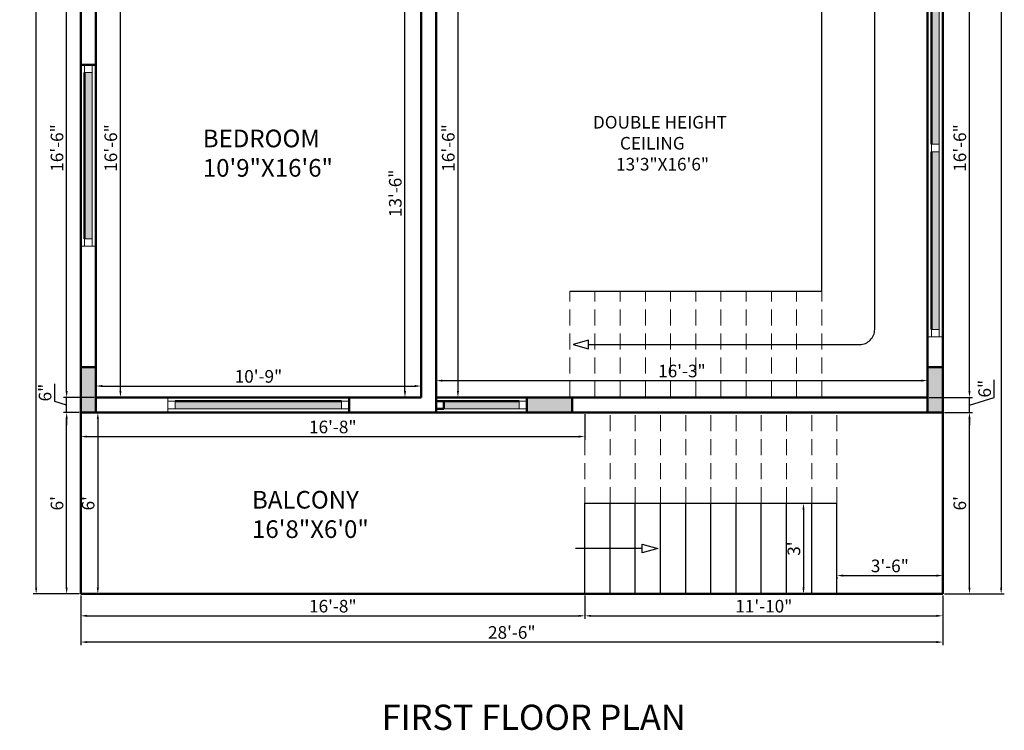
# Model space of a CAD drawing. Units: inches. Extents: x 3064 to 19385, y 846 to 15425.
# Tile 53 of 108: x 6445 to 6835, y 850 to 1132. Entities that reach past the tile are written whole.
import ezdxf

# ---------------------------------------------------------------- set-up
doc = ezdxf.new("R2010")
doc.units = ezdxf.units.IN
doc.linetypes.add('DASHED', pattern=[19.05, 12.7, -6.35])
for name, color, linetype, lineweight in [('A-ANNO-DIMS', 2, 'Continuous', 18), ('A-ANNO-TEXT', 7, 'Continuous', 25), ('A-AREA-IDEN', 3, 'Continuous', 18), ('A-COLS', 1, 'Continuous', 35), ('A-FLOR-STRS', 2, 'Continuous', 25), ('A-FLOR-STRS-OVHD', 2, 'DASHED', 18), ('A-GLAZ', 4, 'Continuous', 18), ('A-WALL', 7, 'Continuous', 50)]:
    doc.layers.add(name, color=color, linetype=linetype, lineweight=lineweight)
doc.styles.get("Standard").update_dxf_attribs({"font": 'arial.ttf'})
doc.dimstyles.new('ISO-25', dxfattribs={"dimtxt": 9, "dimasz": 2.5, "dimexe": 1.25, "dimexo": 0.625, "dimtad": 1, "dimdec": 1, "dimlunit": 3, "dimtxsty": 'Standard', "dimcen": 2.5, "dimadec": 0, "dimazin": 0, "dimtfac": 1, "dimtdec": 1, "dimtmove": 0, "dimatfit": 3, "dimfxl": 1, "dimarcsym": 0})

# ---------------------------------------------------------------- blocks, each defined once
blk = doc.blocks.new('*D135')
at = {"layer": 'A-ANNO-DIMS', "color": 0, "lineweight": -2, "transparency": 16777216}
for p, q in [((6468.41, 976.34), (6462.18, 976.34)), ((6463.43, 906.84), (6463.43, 973.84)), ((6468.41, 904.34), (6462.18, 904.34))]:
    blk.add_line(p, q, dxfattribs=at)
at = {"layer": 'A-ANNO-DIMS', "color": 0, "transparency": 16777216}
for points in [[(6463.02, 973.84), (6463.85, 973.84), (6463.43, 976.34)], [(6463.02, 906.84), (6463.85, 906.84), (6463.43, 904.34)]]:
    blk.add_solid(points, dxfattribs=at)
at = {"layer": 'Defpoints', "color": 0, "transparency": 16777216}
for p in [(6463.43, 976.34), (6469.03, 976.34), (6469.03, 904.34)]:
    blk.add_point(p, dxfattribs=at)
at = {"layer": 'A-ANNO-DIMS', "color": 0, "transparency": 16777216, "insert": (6460.26, 940.34), "char_height": 5, "attachment_point": 5, "rotation": 90}
blk.add_mtext("6'", dxfattribs=at)
blk = doc.blocks.new('*D127')
at = {"layer": 'A-ANNO-DIMS', "color": 0, "lineweight": -2, "transparency": 16777216}
for p, q in [((6458.69, 980.76), (6458.69, 987.79)), ((6463.43, 984.84), (6463.43, 987.34)), ((6463.43, 979.34), (6458.69, 980.76)), ((6474.41, 982.34), (6462.18, 982.34)), ((6463.43, 976.34), (6463.43, 982.34)), ((6463.43, 976.34), (6463.43, 982.34)), ((6468.41, 976.34), (6462.18, 976.34)), ((6463.43, 973.84), (6463.43, 971.34))]:
    blk.add_line(p, q, dxfattribs=at)
at = {"layer": 'A-ANNO-DIMS', "color": 0, "transparency": 16777216}
for points in [[(6463.02, 984.84), (6463.85, 984.84), (6463.43, 982.34)], [(6463.02, 973.84), (6463.85, 973.84), (6463.43, 976.34)]]:
    blk.add_solid(points, dxfattribs=at)
at = {"layer": 'Defpoints', "color": 0, "transparency": 16777216}
for p in [(6463.43, 982.34), (6475.03, 982.34), (6469.03, 976.34)]:
    blk.add_point(p, dxfattribs=at)
at = {"layer": 'A-ANNO-DIMS', "color": 0, "transparency": 16777216, "insert": (6455.52, 984.27), "char_height": 5, "attachment_point": 5, "rotation": 90}
blk.add_mtext('6"', dxfattribs=at)
blk = doc.blocks.new('*D128')
at = {"layer": 'A-ANNO-DIMS', "color": 0, "lineweight": -2, "transparency": 16777216}
for p, q in [((6474.41, 1180.34), (6462.18, 1180.34)), ((6463.43, 984.84), (6463.43, 1177.84)), ((6474.41, 982.34), (6462.18, 982.34))]:
    blk.add_line(p, q, dxfattribs=at)
at = {"layer": 'A-ANNO-DIMS', "color": 0, "transparency": 16777216}
for points in [[(6463.02, 1177.84), (6463.85, 1177.84), (6463.43, 1180.34)], [(6463.02, 984.84), (6463.85, 984.84), (6463.43, 982.34)]]:
    blk.add_solid(points, dxfattribs=at)
at = {"layer": 'Defpoints', "color": 0, "transparency": 16777216}
for p in [(6463.43, 1180.34), (6475.03, 1180.34), (6475.03, 982.34)]:
    blk.add_point(p, dxfattribs=at)
at = {"layer": 'A-ANNO-DIMS', "color": 0, "transparency": 16777216, "insert": (6460.26, 1081.34), "char_height": 5, "attachment_point": 5, "rotation": 90}
blk.add_mtext('16\'-6"', dxfattribs=at)
blk = doc.blocks.new('*D126')
at = {"layer": 'A-ANNO-DIMS', "color": 0, "lineweight": -2, "transparency": 16777216}
for p, q in [((6468.41, 1396.34), (6450.1, 1396.34)), ((6451.35, 906.84), (6451.35, 1393.84)), ((6468.41, 904.34), (6450.1, 904.34))]:
    blk.add_line(p, q, dxfattribs=at)
at = {"layer": 'A-ANNO-DIMS', "color": 0, "transparency": 16777216}
for points in [[(6450.94, 1393.84), (6451.77, 1393.84), (6451.35, 1396.34)], [(6450.94, 906.84), (6451.77, 906.84), (6451.35, 904.34)]]:
    blk.add_solid(points, dxfattribs=at)
at = {"layer": 'Defpoints', "color": 0, "transparency": 16777216}
for p in [(6451.35, 1396.34), (6469.03, 1396.34), (6469.03, 904.34)]:
    blk.add_point(p, dxfattribs=at)
at = {"layer": 'A-ANNO-DIMS', "color": 0, "transparency": 16777216, "insert": (6448.22, 1150.34), "char_height": 5, "attachment_point": 5, "rotation": 90}
blk.add_mtext("41'", dxfattribs=at)
blk = doc.blocks.new('*D115')
at = {"layer": 'A-ANNO-DIMS', "color": 0, "lineweight": -2, "transparency": 16777216}
for p, q in [((6469.03, 903.71), (6469.03, 894.42)), ((6669.03, 903.71), (6669.03, 894.42)), ((6471.53, 895.67), (6666.53, 895.67))]:
    blk.add_line(p, q, dxfattribs=at)
at = {"layer": 'A-ANNO-DIMS', "color": 0, "transparency": 16777216}
for points in [[(6471.53, 896.08), (6471.53, 895.25), (6469.03, 895.67)], [(6666.53, 896.08), (6666.53, 895.25), (6669.03, 895.67)]]:
    blk.add_solid(points, dxfattribs=at)
at = {"layer": 'Defpoints', "color": 0, "transparency": 16777216}
for p in [(6469.03, 904.34), (6669.03, 904.34), (6669.03, 895.67)]:
    blk.add_point(p, dxfattribs=at)
at = {"layer": 'A-ANNO-DIMS', "color": 0, "transparency": 16777216, "insert": (6569.03, 898.85), "char_height": 5, "attachment_point": 5}
blk.add_mtext('16\'-8"', dxfattribs=at)
blk = doc.blocks.new('*D116')
at = {"layer": 'A-ANNO-DIMS', "color": 0, "lineweight": -2, "transparency": 16777216}
for p, q in [((6669.03, 903.71), (6669.03, 894.42)), ((6811.03, 903.71), (6811.03, 894.42)), ((6671.53, 895.67), (6808.53, 895.67))]:
    blk.add_line(p, q, dxfattribs=at)
at = {"layer": 'A-ANNO-DIMS', "color": 0, "transparency": 16777216}
for points in [[(6671.53, 896.08), (6671.53, 895.25), (6669.03, 895.67)], [(6808.53, 896.08), (6808.53, 895.25), (6811.03, 895.67)]]:
    blk.add_solid(points, dxfattribs=at)
at = {"layer": 'Defpoints', "color": 0, "transparency": 16777216}
for p in [(6669.03, 904.34), (6811.03, 904.34), (6811.03, 895.67)]:
    blk.add_point(p, dxfattribs=at)
at = {"layer": 'A-ANNO-DIMS', "color": 0, "transparency": 16777216, "insert": (6740.03, 898.85), "char_height": 5, "attachment_point": 5}
blk.add_mtext('11\'-10"', dxfattribs=at)
blk = doc.blocks.new('*D98')
at = {"layer": 'A-ANNO-DIMS', "color": 0, "lineweight": -2, "transparency": 16777216}
for p, q in [((6469.03, 903.71), (6469.03, 884.01)), ((6811.03, 903.71), (6811.03, 884.01)), ((6808.53, 885.26), (6471.53, 885.26))]:
    blk.add_line(p, q, dxfattribs=at)
at = {"layer": 'A-ANNO-DIMS', "color": 0, "transparency": 16777216}
for points in [[(6471.53, 885.67), (6471.53, 884.84), (6469.03, 885.26)], [(6808.53, 885.67), (6808.53, 884.84), (6811.03, 885.26)]]:
    blk.add_solid(points, dxfattribs=at)
at = {"layer": 'Defpoints', "color": 0, "transparency": 16777216}
for p in [(6469.03, 904.34), (6811.03, 904.34), (6469.03, 885.26)]:
    blk.add_point(p, dxfattribs=at)
at = {"layer": 'A-ANNO-DIMS', "color": 0, "transparency": 16777216, "insert": (6640.03, 888.43), "char_height": 5, "attachment_point": 5}
blk.add_mtext('28\'-6"', dxfattribs=at)
blk = doc.blocks.new('*D117')
at = {"layer": 'A-ANNO-DIMS', "color": 0, "lineweight": -2, "transparency": 16777216}
for p, q in [((6811.66, 976.34), (6822.87, 976.34)), ((6821.62, 906.84), (6821.62, 973.84)), ((6811.66, 904.34), (6822.87, 904.34))]:
    blk.add_line(p, q, dxfattribs=at)
at = {"layer": 'A-ANNO-DIMS', "color": 0, "transparency": 16777216}
for points in [[(6821.2, 973.84), (6822.03, 973.84), (6821.62, 976.34)], [(6821.2, 906.84), (6822.03, 906.84), (6821.62, 904.34)]]:
    blk.add_solid(points, dxfattribs=at)
at = {"layer": 'Defpoints', "color": 0, "transparency": 16777216}
for p in [(6811.03, 976.34), (6821.62, 976.34), (6811.03, 904.34)]:
    blk.add_point(p, dxfattribs=at)
at = {"layer": 'A-ANNO-DIMS', "color": 0, "transparency": 16777216, "insert": (6818.44, 940.34), "char_height": 5, "attachment_point": 5, "rotation": 90}
blk.add_mtext("6'", dxfattribs=at)
blk = doc.blocks.new('*D118')
at = {"layer": 'A-ANNO-DIMS', "color": 0, "lineweight": -2, "transparency": 16777216}
for p, q in [((6831.46, 982.29), (6831.46, 989.32)), ((6821.62, 984.84), (6821.62, 987.34)), ((6805.66, 982.34), (6822.87, 982.34)), ((6821.62, 976.34), (6821.62, 982.34)), ((6821.62, 976.34), (6821.62, 982.34)), ((6821.62, 979.34), (6831.46, 982.29)), ((6811.66, 976.34), (6822.87, 976.34)), ((6821.62, 973.84), (6821.62, 971.34))]:
    blk.add_line(p, q, dxfattribs=at)
at = {"layer": 'A-ANNO-DIMS', "color": 0, "transparency": 16777216}
for points in [[(6821.2, 984.84), (6822.03, 984.84), (6821.62, 982.34)], [(6821.2, 973.84), (6822.03, 973.84), (6821.62, 976.34)]]:
    blk.add_solid(points, dxfattribs=at)
at = {"layer": 'Defpoints', "color": 0, "transparency": 16777216}
for p in [(6805.03, 982.34), (6821.62, 982.34), (6811.03, 976.34)]:
    blk.add_point(p, dxfattribs=at)
at = {"layer": 'A-ANNO-DIMS', "color": 0, "transparency": 16777216, "insert": (6828.28, 985.81), "char_height": 5, "attachment_point": 5, "rotation": 90}
blk.add_mtext('6"', dxfattribs=at)
blk = doc.blocks.new('*D119')
at = {"layer": 'A-ANNO-DIMS', "color": 0, "lineweight": -2, "transparency": 16777216}
for p, q in [((6811.66, 1180.34), (6822.87, 1180.34)), ((6821.62, 984.84), (6821.62, 1177.84)), ((6805.66, 982.34), (6822.87, 982.34))]:
    blk.add_line(p, q, dxfattribs=at)
at = {"layer": 'A-ANNO-DIMS', "color": 0, "transparency": 16777216}
for points in [[(6821.2, 1177.84), (6822.03, 1177.84), (6821.62, 1180.34)], [(6821.2, 984.84), (6822.03, 984.84), (6821.62, 982.34)]]:
    blk.add_solid(points, dxfattribs=at)
at = {"layer": 'Defpoints', "color": 0, "transparency": 16777216}
for p in [(6811.03, 1180.34), (6821.62, 1180.34), (6805.03, 982.34)]:
    blk.add_point(p, dxfattribs=at)
at = {"layer": 'A-ANNO-DIMS', "color": 0, "transparency": 16777216, "insert": (6818.44, 1081.34), "char_height": 5, "attachment_point": 5, "rotation": 90}
blk.add_mtext('16\'-6"', dxfattribs=at)
blk = doc.blocks.new('*D104')
at = {"layer": 'A-ANNO-DIMS', "color": 0, "lineweight": -2, "transparency": 16777216}
for p, q in [((6811.66, 1396.34), (6835.44, 1396.34)), ((6834.19, 1393.84), (6834.19, 906.84)), ((6811.66, 904.34), (6835.44, 904.34))]:
    blk.add_line(p, q, dxfattribs=at)
at = {"layer": 'A-ANNO-DIMS', "color": 0, "transparency": 16777216}
for points in [[(6833.77, 1393.84), (6834.6, 1393.84), (6834.19, 1396.34)], [(6833.77, 906.84), (6834.6, 906.84), (6834.19, 904.34)]]:
    blk.add_solid(points, dxfattribs=at)
at = {"layer": 'Defpoints', "color": 0, "transparency": 16777216}
for p in [(6811.03, 1396.34), (6811.03, 904.34), (6834.19, 904.34)]:
    blk.add_point(p, dxfattribs=at)
at = {"layer": 'A-ANNO-DIMS', "color": 0, "transparency": 16777216, "insert": (6831.05, 1150.34), "char_height": 5, "attachment_point": 5, "rotation": 90}
blk.add_mtext("41'", dxfattribs=at)
blk = doc.blocks.new('*D181')
at = {"layer": 'A-ANNO-DIMS', "color": 0, "lineweight": -2, "transparency": 16777216}
for p, q in [((6469.03, 975.71), (6469.03, 965.55)), ((6669.03, 975.71), (6669.03, 965.55)), ((6471.53, 966.8), (6666.53, 966.8))]:
    blk.add_line(p, q, dxfattribs=at)
at = {"layer": 'A-ANNO-DIMS', "color": 0, "transparency": 16777216}
for points in [[(6471.53, 967.22), (6471.53, 966.39), (6469.03, 966.8)], [(6666.53, 967.22), (6666.53, 966.39), (6669.03, 966.8)]]:
    blk.add_solid(points, dxfattribs=at)
at = {"layer": 'Defpoints', "color": 0, "transparency": 16777216}
for p in [(6469.03, 976.34), (6669.03, 976.34), (6669.03, 966.8)]:
    blk.add_point(p, dxfattribs=at)
at = {"layer": 'A-ANNO-DIMS', "color": 0, "transparency": 16777216, "insert": (6569.03, 969.98), "char_height": 5, "attachment_point": 5}
blk.add_mtext('16\'-8"', dxfattribs=at)
blk = doc.blocks.new('*D182')
at = {"layer": 'A-ANNO-DIMS', "color": 0, "lineweight": -2, "transparency": 16777216}
for p, q in [((6469.66, 976.34), (6477.06, 976.34)), ((6475.81, 973.84), (6475.81, 906.84)), ((6469.66, 904.34), (6477.06, 904.34))]:
    blk.add_line(p, q, dxfattribs=at)
at = {"layer": 'A-ANNO-DIMS', "color": 0, "transparency": 16777216}
for points in [[(6475.39, 973.84), (6476.23, 973.84), (6475.81, 976.34)], [(6475.39, 906.84), (6476.23, 906.84), (6475.81, 904.34)]]:
    blk.add_solid(points, dxfattribs=at)
at = {"layer": 'Defpoints', "color": 0, "transparency": 16777216}
for p in [(6469.03, 976.34), (6469.03, 904.34), (6475.81, 904.34)]:
    blk.add_point(p, dxfattribs=at)
at = {"layer": 'A-ANNO-DIMS', "color": 0, "transparency": 16777216, "insert": (6472.63, 940.34), "char_height": 5, "attachment_point": 5, "rotation": 90}
blk.add_mtext("6'", dxfattribs=at)
blk = doc.blocks.new('*D183')
at = {"layer": 'A-ANNO-DIMS', "color": 0, "lineweight": -2, "transparency": 16777216}
for p, q in [((6769.03, 911.03), (6769.03, 910.4)), ((6771.53, 911.65), (6808.53, 911.65)), ((6811.03, 912.28), (6811.03, 912.9))]:
    blk.add_line(p, q, dxfattribs=at)
at = {"layer": 'A-ANNO-DIMS', "color": 0, "transparency": 16777216}
for points in [[(6771.53, 912.07), (6771.53, 911.23), (6769.03, 911.65)], [(6808.53, 912.07), (6808.53, 911.23), (6811.03, 911.65)]]:
    blk.add_solid(points, dxfattribs=at)
at = {"layer": 'Defpoints', "color": 0, "transparency": 16777216}
for p in [(6769.03, 911.65), (6811.03, 911.65), (6811.03, 911.65)]:
    blk.add_point(p, dxfattribs=at)
at = {"layer": 'A-ANNO-DIMS', "color": 0, "transparency": 16777216, "insert": (6790.03, 914.83), "char_height": 5, "attachment_point": 5}
blk.add_mtext('3\'-6"', dxfattribs=at)
blk = doc.blocks.new('*D184')
at = {"layer": 'A-ANNO-DIMS', "color": 0, "lineweight": -2, "transparency": 16777216}
for p, q in [((6754.21, 940.34), (6757.03, 940.34)), ((6755.78, 937.84), (6755.78, 906.84)), ((6754.21, 904.34), (6757.03, 904.34))]:
    blk.add_line(p, q, dxfattribs=at)
at = {"layer": 'A-ANNO-DIMS', "color": 0, "transparency": 16777216}
for points in [[(6755.36, 937.84), (6756.19, 937.84), (6755.78, 940.34)], [(6755.36, 906.84), (6756.19, 906.84), (6755.78, 904.34)]]:
    blk.add_solid(points, dxfattribs=at)
at = {"layer": 'Defpoints', "color": 0, "transparency": 16777216}
for p in [(6753.58, 940.34), (6753.58, 904.34), (6755.78, 904.34)]:
    blk.add_point(p, dxfattribs=at)
at = {"layer": 'A-ANNO-DIMS', "color": 0, "transparency": 16777216, "insert": (6752.6, 922.34), "char_height": 5, "attachment_point": 5, "rotation": 90}
blk.add_mtext("3'", dxfattribs=at)
blk = doc.blocks.new('*D187')
at = {"layer": 'A-ANNO-DIMS', "color": 0, "lineweight": -2, "transparency": 16777216}
for p, q in [((6475.03, 982.96), (6475.03, 988.12)), ((6477.53, 986.87), (6601.53, 986.87)), ((6604.03, 982.96), (6604.03, 988.12))]:
    blk.add_line(p, q, dxfattribs=at)
at = {"layer": 'A-ANNO-DIMS', "color": 0, "transparency": 16777216}
for points in [[(6477.53, 987.29), (6477.53, 986.45), (6475.03, 986.87)], [(6601.53, 987.29), (6601.53, 986.45), (6604.03, 986.87)]]:
    blk.add_solid(points, dxfattribs=at)
at = {"layer": 'Defpoints', "color": 0, "transparency": 16777216}
for p in [(6604.03, 986.87), (6475.03, 982.34), (6604.03, 982.34)]:
    blk.add_point(p, dxfattribs=at)
at = {"layer": 'A-ANNO-DIMS', "color": 0, "transparency": 16777216, "insert": (6539.53, 990.05), "char_height": 5, "attachment_point": 5}
blk.add_mtext('10\'-9"', dxfattribs=at)
blk = doc.blocks.new('*D188')
at = {"layer": 'A-ANNO-DIMS', "color": 0, "lineweight": -2, "transparency": 16777216}
for p, q in [((6475.66, 1180.34), (6486.03, 1180.34)), ((6484.78, 984.84), (6484.78, 1177.84)), ((6475.66, 982.34), (6486.03, 982.34))]:
    blk.add_line(p, q, dxfattribs=at)
at = {"layer": 'A-ANNO-DIMS', "color": 0, "transparency": 16777216}
for points in [[(6484.37, 1177.84), (6485.2, 1177.84), (6484.78, 1180.34)], [(6484.37, 984.84), (6485.2, 984.84), (6484.78, 982.34)]]:
    blk.add_solid(points, dxfattribs=at)
at = {"layer": 'Defpoints', "color": 0, "transparency": 16777216}
for p in [(6475.03, 1180.34), (6484.78, 1180.34), (6475.03, 982.34)]:
    blk.add_point(p, dxfattribs=at)
at = {"layer": 'A-ANNO-DIMS', "color": 0, "transparency": 16777216, "insert": (6481.6, 1081.34), "char_height": 5, "attachment_point": 5, "rotation": 90}
blk.add_mtext('16\'-6"', dxfattribs=at)
blk = doc.blocks.new('*D192')
at = {"layer": 'A-ANNO-DIMS', "color": 0, "lineweight": -2, "transparency": 16777216}
for p, q in [((6603.41, 1144.34), (6596.41, 1144.34)), ((6597.66, 984.84), (6597.66, 1141.84)), ((6603.41, 982.34), (6596.41, 982.34))]:
    blk.add_line(p, q, dxfattribs=at)
at = {"layer": 'A-ANNO-DIMS', "color": 0, "transparency": 16777216}
for points in [[(6597.25, 1141.84), (6598.08, 1141.84), (6597.66, 1144.34)], [(6597.25, 984.84), (6598.08, 984.84), (6597.66, 982.34)]]:
    blk.add_solid(points, dxfattribs=at)
at = {"layer": 'Defpoints', "color": 0, "transparency": 16777216}
for p in [(6597.66, 1144.34), (6604.03, 1144.34), (6604.03, 982.34)]:
    blk.add_point(p, dxfattribs=at)
at = {"layer": 'A-ANNO-DIMS', "color": 0, "transparency": 16777216, "insert": (6594.48, 1063.34), "char_height": 5, "attachment_point": 5, "rotation": 90}
blk.add_mtext('13\'-6"', dxfattribs=at)
blk = doc.blocks.new('*D216')
at = {"layer": 'A-ANNO-DIMS', "color": 0, "lineweight": -2, "transparency": 16777216}
for p, q in [((6610.66, 1180.34), (6619.92, 1180.34)), ((6618.67, 1177.84), (6618.67, 984.84)), ((6610.66, 982.34), (6619.92, 982.34))]:
    blk.add_line(p, q, dxfattribs=at)
at = {"layer": 'A-ANNO-DIMS', "color": 0, "transparency": 16777216}
for points in [[(6618.26, 1177.84), (6619.09, 1177.84), (6618.67, 1180.34)], [(6618.26, 984.84), (6619.09, 984.84), (6618.67, 982.34)]]:
    blk.add_solid(points, dxfattribs=at)
at = {"layer": 'Defpoints', "color": 0, "transparency": 16777216}
for p in [(6610.03, 1180.34), (6610.03, 982.34), (6618.67, 982.34)]:
    blk.add_point(p, dxfattribs=at)
at = {"layer": 'A-ANNO-DIMS', "color": 0, "transparency": 16777216, "insert": (6615.5, 1081.34), "char_height": 5, "attachment_point": 5, "rotation": 90}
blk.add_mtext('16\'-6"', dxfattribs=at)
blk = doc.blocks.new('*D217')
at = {"layer": 'A-ANNO-DIMS', "color": 0, "lineweight": -2, "transparency": 16777216}
for p, q in [((6610.03, 982.96), (6610.03, 990.26)), ((6612.53, 989.01), (6802.53, 989.01)), ((6805.03, 982.96), (6805.03, 990.26))]:
    blk.add_line(p, q, dxfattribs=at)
at = {"layer": 'A-ANNO-DIMS', "color": 0, "transparency": 16777216}
for points in [[(6612.53, 989.43), (6612.53, 988.6), (6610.03, 989.01)], [(6802.53, 989.43), (6802.53, 988.6), (6805.03, 989.01)]]:
    blk.add_solid(points, dxfattribs=at)
at = {"layer": 'Defpoints', "color": 0, "transparency": 16777216}
for p in [(6805.03, 989.01), (6610.03, 982.34), (6805.03, 982.34)]:
    blk.add_point(p, dxfattribs=at)
at = {"layer": 'A-ANNO-DIMS', "color": 0, "transparency": 16777216, "insert": (6707.53, 992.19), "char_height": 5, "attachment_point": 5}
blk.add_mtext('16\'-3"', dxfattribs=at)
blk = doc.blocks.new('WIN-1800-PAIR')
h = blk.add_hatch(color=256)
h.dxf.hatch_style = 1
h.paths.add_polyline_path([(0, 0), (3, 0), (3, 70.5), (0, 70.5)])
h.paths.add_polyline_path([(3, 144), (0, 144), (0, 73.5), (3, 73.5)])
blk.add_line((3, 144), (3, 73.5))
blk.add_lwpolyline([(3, 144), (0, 144), (0, 147), (3, 147)], close=True)
blk = doc.blocks.new('WIN-900')
blk.add_line((0, 0), (30, 0))
blk.add_lwpolyline([(30, 0), (30, 3), (33, 3), (33, 0)], close=True)
blk = doc.blocks.new('WIN-2000')
blk.add_line((3, 0), (3, 70.5))
blk.add_lwpolyline([(3, 70.5), (0, 70.5), (0, 73.5), (3, 73.5)], close=True)
blk = doc.blocks.new('WIN-1900')
blk.add_line((3, 0), (3, 66))
blk.add_lwpolyline([(3, 66), (0, 66), (0, 69), (3, 69)], close=True)

msp = doc.modelspace()

# ---------------------------------------------------------------- hatches: boundary and pattern name
at = {"layer": 'A-COLS'}
h = msp.add_hatch(color=256, dxfattribs=at)
h.dxf.hatch_style = 1
h.paths.add_polyline_path([(6469.03, 976.34), (6475.03, 976.34), (6475.03, 994.34), (6469.03, 994.34)])
h = msp.add_hatch(color=256, dxfattribs=at)
h.dxf.hatch_style = 1
h.paths.add_polyline_path([(6805.03, 976.34), (6811.03, 976.34), (6811.03, 994.34), (6805.03, 994.34)])
h = msp.add_hatch(color=256, dxfattribs=at)
h.dxf.hatch_style = 1
h.paths.add_polyline_path([(6664.03, 976.34), (6664.03, 982.34), (6646.03, 982.34), (6646.03, 976.34)])
at = {"layer": 'A-GLAZ'}
h = msp.add_hatch(color=256, dxfattribs=at)
h.dxf.hatch_style = 1
h.paths.add_polyline_path([(6470.53, 1045.34), (6473.53, 1045.34), (6473.53, 1111.34), (6470.53, 1111.34)])
h = msp.add_hatch(color=256, dxfattribs=at)
h.dxf.hatch_style = 1
h.paths.add_polyline_path([(6506.53, 980.84), (6506.53, 977.84), (6572.53, 977.84), (6572.53, 980.84)])
h = msp.add_hatch(color=256, dxfattribs=at)
h.dxf.hatch_style = 1
h.paths.add_polyline_path([(6613.03, 980.84), (6613.03, 977.84), (6643.03, 977.84), (6643.03, 980.84)])

# ---------------------------------------------------------------- linework, layer by layer
at = {"layer": 'A-FLOR-STRS'}
for p, q in [((6763.03, 1024.34), (6763.03, 1180.34)), ((6763.03, 1024.34), (6663.03, 1024.34)), ((6669.03, 904.34), (6669.03, 940.34)), ((6669.03, 940.34), (6769.03, 940.34)), ((6679.03, 904.34), (6679.03, 940.34)), ((6689.03, 904.34), (6689.03, 940.34)), ((6699.03, 904.34), (6699.03, 940.34)), ((6709.03, 904.34), (6709.03, 940.34)), ((6719.03, 904.34), (6719.03, 940.34)), ((6729.03, 904.34), (6729.03, 940.34)), ((6739.03, 904.34), (6739.03, 940.34)), ((6749.03, 904.34), (6749.03, 940.34)), ((6759.03, 904.34), (6759.03, 940.34)), ((6769.03, 904.34), (6769.03, 940.34)), ((6691.74, 922.34), (6665.34, 922.34))]:
    msp.add_line(p, q, dxfattribs=at)
msp.add_lwpolyline([(6670.52, 1003.34), (6778.03, 1003.34, 0.414214), (6784.03, 1009.34), (6784.03, 1153.34, 0.414214), (6778.03, 1159.34), (6651.03, 1159.34)], format="xyb", dxfattribs=at)
for points in [[(6664.33, 1003.34), (6670.52, 1001.61), (6670.52, 1005.07)], [(6697.93, 922.34), (6691.74, 920.61), (6691.74, 924.07)]]:
    msp.add_lwpolyline(points, close=True, dxfattribs=at)
at = {"layer": 'A-FLOR-STRS-OVHD', "ltscale": 0.5}
for p, q in [((6663.03, 982.34), (6663.03, 1024.34)), ((6673.03, 982.34), (6673.03, 1024.34)), ((6683.03, 982.34), (6683.03, 1024.34)), ((6693.03, 982.34), (6693.03, 1024.34)), ((6703.03, 982.34), (6703.03, 1024.34)), ((6713.03, 982.34), (6713.03, 1024.34)), ((6723.03, 982.34), (6723.03, 1024.34)), ((6733.03, 982.34), (6733.03, 1024.34)), ((6743.03, 982.34), (6743.03, 1024.34)), ((6753.03, 982.34), (6753.03, 1024.34)), ((6763.03, 982.34), (6763.03, 1024.34)), ((6669.03, 940.34), (6669.03, 976.34)), ((6679.03, 940.34), (6679.03, 976.34)), ((6689.03, 940.34), (6689.03, 976.34)), ((6699.03, 940.34), (6699.03, 976.34)), ((6709.03, 940.34), (6709.03, 976.34)), ((6719.03, 940.34), (6719.03, 976.34)), ((6729.03, 940.34), (6729.03, 976.34)), ((6739.03, 940.34), (6739.03, 976.34)), ((6749.03, 940.34), (6749.03, 976.34)), ((6759.03, 940.34), (6759.03, 976.34)), ((6769.03, 940.34), (6769.03, 976.34))]:
    msp.add_line(p, q, dxfattribs=at)
at = {"layer": 'A-GLAZ'}
for p, q in [((6475.03, 1042.34), (6469.03, 1042.34)), ((6811.03, 1006.34), (6805.03, 1006.34)), ((6811.03, 1006.34), (6805.03, 1006.34)), ((6503.53, 976.34), (6503.53, 982.34))]:
    msp.add_line(p, q, dxfattribs=at)
for points in [[(6473.53, 1042.34), (6470.53, 1042.34), (6470.53, 1045.34), (6473.53, 1045.34)], [(6809.53, 1006.34), (6806.53, 1006.34), (6806.53, 1009.34), (6809.53, 1009.34)], [(6503.53, 977.84), (6503.53, 980.84), (6506.53, 980.84), (6506.53, 977.84)]]:
    msp.add_lwpolyline(points, close=True, dxfattribs=at)
at = {"layer": 'A-WALL'}
for p, q in [((6469.03, 1396.34), (6469.03, 976.34)), ((6811.03, 904.34), (6811.03, 1396.34)), ((6475.03, 1180.34), (6475.03, 982.34)), ((6805.03, 982.34), (6805.03, 1180.34)), ((6806.53, 1153.34), (6806.53, 1082.84)), ((6604.03, 1144.34), (6604.03, 982.34)), ((6610.03, 1144.34), (6610.03, 976.34)), ((6475.03, 1114.34), (6469.03, 1114.34)), ((6470.53, 1045.34), (6470.53, 1111.34)), ((6806.53, 1009.34), (6806.53, 1079.84)), ((6604.03, 982.34), (6475.03, 982.34)), ((6506.53, 980.84), (6572.53, 980.84)), ((6575.53, 976.34), (6575.53, 982.34)), ((6805.03, 982.34), (6610.03, 982.34)), ((6610.03, 976.34), (6610.03, 982.34)), ((6613.03, 980.84), (6643.03, 980.84)), ((6646.03, 976.34), (6646.03, 982.34)), ((6646.03, 976.34), (6646.03, 982.34)), ((6811.03, 976.34), (6469.03, 976.34)), ((6475.03, 976.34), (6469.03, 976.34)), ((6469.03, 976.34), (6469.03, 904.34)), ((6469.03, 904.34), (6811.03, 904.34))]:
    msp.add_line(p, q, dxfattribs=at)
for points in [[(6475.03, 976.34), (6475.03, 994.34), (6469.03, 994.34), (6469.03, 976.34)], [(6811.03, 976.34), (6811.03, 994.34), (6805.03, 994.34), (6805.03, 976.34)], [(6610.03, 977.84), (6610.03, 980.84), (6613.03, 980.84), (6613.03, 977.84)], [(6664.03, 982.34), (6646.03, 982.34), (6646.03, 976.34), (6664.03, 976.34)]]:
    msp.add_lwpolyline(points, close=True, dxfattribs=at)

# ---------------------------------------------------------------- block references
at = {"layer": 'A-GLAZ'}
for name, p in [('WIN-1800-PAIR', (6806.53, 1009.34)), ('WIN-1900', (6470.53, 1045.34)), ('WIN-2000', (6806.53, 1009.34)), ('WIN-900', (6613.03, 977.84))]:
    msp.add_blockref(name, p, dxfattribs=at)
at = {"layer": 'A-GLAZ', "rotation": 269.9999999999995}
msp.add_blockref('WIN-1900', (6506.53, 980.84), dxfattribs=at)

# ---------------------------------------------------------------- texts
at = {"layer": 'A-ANNO-TEXT', "insert": (6588.38, 860.41), "char_height": 10, "attachment_point": 1}
msp.add_mtext_dynamic_manual_height_columns('FIRST FLOOR PLAN', width=200.9739, gutter_width=12.5, heights=[0], dxfattribs=at)
at = {"layer": 'A-AREA-IDEN', "attachment_point": 1}
for s, width, insert, char_height in [('DOUBLE HEIGHT \\P       CEILING            \\P      13\'3"X16\'6"', 57.0817, (6672.24, 1094.07), 5), ('BEDROOM\\P10\'9"X16\'6"', 67.5924, (6517.45, 1088.62), 7), ('BALCONY\\P16\'8"X6\'0"', 67.5924, (6536.97, 945.24), 7)]:
    msp.add_mtext_dynamic_manual_height_columns(s, width=width, gutter_width=12.5, heights=[0], dxfattribs=dict(at, insert=insert, char_height=char_height))

# ---------------------------------------------------------------- dimensions: what is measured, and where the dimension line sits
at = {"layer": 'A-ANNO-DIMS'}
for base, p1, p2, override, picture, middle in [((6451.35, 1396.34), (6469.03, 904.34), (6469.03, 1396.34), {"dimtxt": 5, "dimclrd": 0, "dimclre": 0, "dimclrt": 0}, '*D126', (6448.22, 1150.34)), ((6834.19, 904.34), (6811.03, 1396.34), (6811.03, 904.34), {"dimtxt": 5, "dimclrd": 0, "dimclre": 0, "dimclrt": 0}, '*D104', (6831.05, 1150.34)), ((6463.43, 1180.34), (6475.03, 982.34), (6475.03, 1180.34), {"dimtxt": 5, "dimclrd": 0, "dimclre": 0, "dimclrt": 0, "dimtmove": 1}, '*D128', (6460.26, 1081.34)), ((6484.78, 1180.34), (6475.03, 982.34), (6475.03, 1180.34), {"dimtxt": 5, "dimclrd": 0, "dimclre": 0, "dimclrt": 0}, '*D188', (6481.6, 1081.34)), ((6618.67, 982.34), (6610.03, 1180.34), (6610.03, 982.34), {"dimtxt": 5, "dimclrd": 0, "dimclre": 0, "dimclrt": 0}, '*D216', (6615.5, 1081.34)), ((6821.62, 1180.34), (6805.03, 982.34), (6811.03, 1180.34), {"dimtxt": 5, "dimclrd": 0, "dimclre": 0, "dimclrt": 0, "dimtmove": 1}, '*D119', (6818.44, 1081.34)), ((6597.66, 1144.34), (6604.03, 982.34), (6604.03, 1144.34), {"dimtxt": 5, "dimclrd": 0, "dimclre": 0, "dimclrt": 0}, '*D192', (6594.48, 1063.34)), ((6821.62, 982.34), (6811.03, 976.34), (6805.03, 982.34), {"dimtxt": 5, "dimclrd": 0, "dimclre": 0, "dimclrt": 0, "dimtmove": 1}, '*D118', (6828.28, 982.92)), ((6463.43, 982.34), (6469.03, 976.34), (6475.03, 982.34), {"dimtxt": 5, "dimclrd": 0, "dimclre": 0, "dimclrt": 0, "dimtmove": 1}, '*D127', (6455.52, 981.39)), ((6463.43, 976.34), (6469.03, 904.34), (6469.03, 976.34), {"dimtxt": 5, "dimclrd": 0, "dimclre": 0, "dimclrt": 0}, '*D135', (6460.26, 940.34)), ((6475.81, 904.34), (6469.03, 976.34), (6469.03, 904.34), {"dimtxt": 5, "dimclrd": 0, "dimclre": 0, "dimclrt": 0}, '*D182', (6472.63, 940.34)), ((6821.62, 976.34), (6811.03, 904.34), (6811.03, 976.34), {"dimtxt": 5, "dimclrd": 0, "dimclre": 0, "dimclrt": 0}, '*D117', (6818.44, 940.34)), ((6755.78, 904.34), (6753.58, 940.34), (6753.58, 904.34), {"dimtxt": 5, "dimclrd": 0, "dimclre": 0, "dimclrt": 0}, '*D184', (6752.6, 922.34))]:
    dim = msp.add_linear_dim(base=base, p1=p1, p2=p2, angle=90, dimstyle='ISO-25', override=override, dxfattribs=at)
    dim.commit()
    dim.dimension.update_dxf_attribs({"geometry": picture, "text_midpoint": middle})
for base, p1, p2, override, picture, middle in [((6604.03, 986.87), (6475.03, 982.34), (6604.03, 982.34), {"dimtxt": 5, "dimclrd": 0, "dimclre": 0, "dimclrt": 0}, '*D187', (6539.53, 990.05)), ((6805.03, 989.01), (6610.03, 982.34), (6805.03, 982.34), {"dimtxt": 5, "dimclrd": 0, "dimclre": 0, "dimclrt": 0}, '*D217', (6707.53, 992.19)), ((6669.03, 966.8), (6469.03, 976.34), (6669.03, 976.34), {"dimtxt": 5, "dimclrd": 0, "dimclre": 0, "dimclrt": 0}, '*D181', (6569.03, 969.98)), ((6811.03, 911.65), (6769.03, 911.65), (6811.03, 911.65), {"dimtxt": 5, "dimclrd": 0, "dimclre": 0, "dimclrt": 0}, '*D183', (6790.03, 914.83)), ((6669.03, 895.67), (6469.03, 904.34), (6669.03, 904.34), {"dimtxt": 5, "dimclrd": 0, "dimclre": 0, "dimclrt": 0}, '*D115', (6569.03, 898.85)), ((6469.03, 885.26), (6811.03, 904.34), (6469.03, 904.34), {"dimtxt": 5, "dimclrd": 0, "dimclre": 0, "dimclrt": 0}, '*D98', (6640.03, 888.43)), ((6811.03, 895.67), (6669.03, 904.34), (6811.03, 904.34), {"dimtxt": 5, "dimclrd": 0, "dimclre": 0, "dimclrt": 0, "dimtmove": 1}, '*D116', (6740.03, 898.85))]:
    dim = msp.add_linear_dim(base=base, p1=p1, p2=p2, dimstyle='ISO-25', override=override, dxfattribs=at)
    dim.commit()
    dim.dimension.update_dxf_attribs({"geometry": picture, "text_midpoint": middle})

doc.saveas('drawing.dxf')
